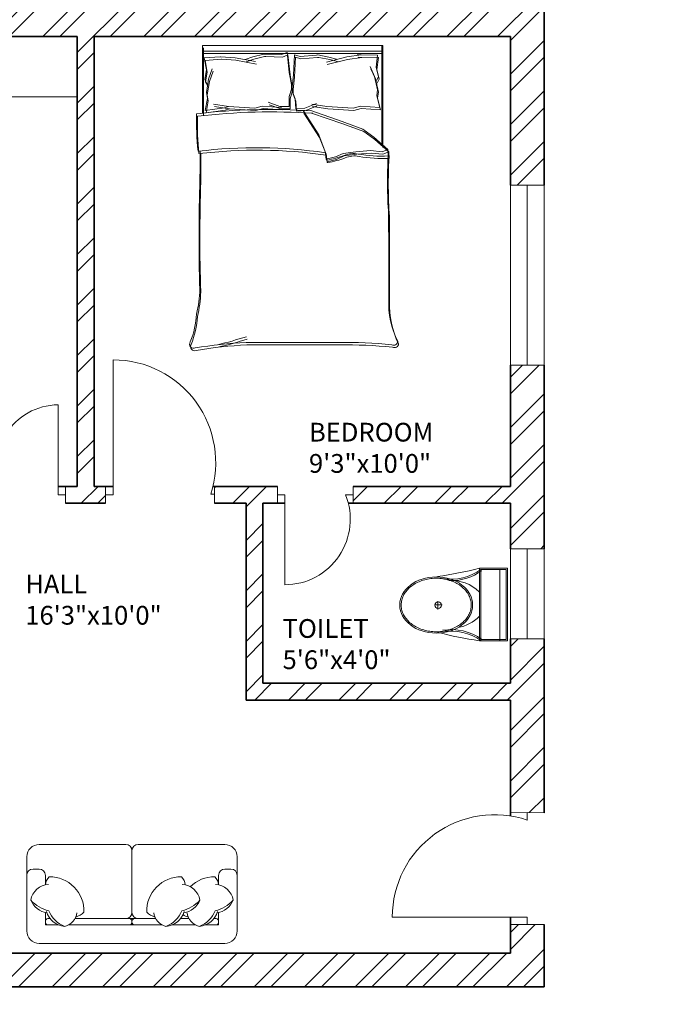
# Model space of a CAD drawing. Units: inches. Extents: x 2552 to 3217, y 1417 to 2737.
# Tile 3 of 25: x 2709 to 2885, y 1622 to 1885. Entities that reach past the tile are written whole.
import ezdxf

# ---------------------------------------------------------------- set-up
doc = ezdxf.new("R2010")
doc.units = ezdxf.units.IN
for name, color, linetype, lineweight in [('A-ANNO-DIMS', 2, 'Continuous', 18), ('A-AREA-IDEN', 7, 'Continuous', 18), ('A-DOOR', 21, 'Continuous', 18), ('A-FLOR-CASE', 9, 'Continuous', 18), ('A-FLOR-FIXT', 8, 'Continuous', 18), ('A-FURN', 8, 'Continuous', 13), ('A-GLAZ', 161, 'Continuous', 18), ('A-WALL', 7, 'Continuous', 35), ('A-WALL-PATT', 217, 'Continuous', 13)]:
    doc.layers.add(name, color=color, linetype=linetype, lineweight=lineweight)
doc.styles.get("Standard").update_dxf_attribs({"font": 'arial.ttf'})
doc.dimstyles.get("Standard").update_dxf_attribs({"dimtxt": 0.18, "dimasz": 0.18, "dimexe": 0.18, "dimexo": 0.0625, "dimgap": 0.09, "dimtad": 0, "dimtih": 1, "dimtoh": 1, "dimdec": 4, "dimzin": 0, "dimdsep": 46, "dimtxsty": 'Standard', "dimcen": 0.09, "dimadec": 0, "dimazin": 0, "dimtfac": 1, "dimtdec": 4, "dimtofl": 0, "dimtmove": 0, "dimatfit": 3, "dimfxl": 1, "dimtolj": 1, "dimtzin": 0, "dimarcsym": 0})

# ---------------------------------------------------------------- blocks, each defined once
blk = doc.blocks.new('A$C31115884')
for p, q in [((283.1, 497.7), (223.4, 497.7)), ((257.5, 466.4), (257.5, 523.2)), ((0, 200), (0, 0)), ((520, 200), (0, 200)), ((10, 190), (10, 10)), ((510, 190), (10, 190)), ((510, 10), (510, 190)), ((520, 0), (520, 200)), ((510, 54.5), (0, 54.5)), ((10, 10), (510, 10)), ((0, 0), (520, 0))]:
    blk.add_line(p, q)
blk.add_circle((255.6, 496.4), 23.6)
for centre, radius, start, end in [((2777.7, -204.6), 2807, 165.4549, 171.71327), ((3237, 905), 2807, 188.28673, 194.5451), ((-294.5, 403.3), 364.7, 324.20913, 9.34987), ((-294.5, 403.3), 374.7, 324.20913, 9.34987), ((805.8, 403.3), 364.7, 170.65013, 215.79087), ((383.6, 406.2), 293.5, 190.27735, 224.15636), ((139.5, 406.2), 293.5, 315.84364, 2.65635), ((805.8, 403.3), 374.7, 179.20365, 215.79087)]:
    blk.add_arc(centre, radius, start, end)
blk.add_ellipse((256.2, 509.9), major_axis=(0, -260.7), ratio=0.772727)
blk.add_open_spline([(256.2, 259.2), (263.1, 259.2), (270, 259.7), (287.8, 262.3), (298.7, 265.1), (319.9, 273.1), (330.2, 278.4), (350.1, 291.1), (359.7, 298.7), (377.7, 315.9), (386.2, 325.5), (401.7, 346.6), (408.8, 358.1), (421.3, 382.5), (426.8, 395.5), (435.9, 422.4), (439.5, 436.4), (444.8, 465.1), (446.5, 479.7), (447.9, 509.2), (447.6, 524), (445, 553.3), (442.7, 567.8), (436.3, 596), (432.1, 609.7), (421.9, 636), (416, 648.6), (402.5, 672.1), (395, 683), (378.6, 703), (369.8, 712.1), (351.1, 728), (341.3, 734.8), (320.9, 746.2), (310.4, 750.7), (288.9, 757.3), (278, 759.4), (256, 761), (245, 760.6), (223.1, 757.2), (212.3, 754.3), (191.1, 746.1), (180.8, 740.7), (160.9, 727.8), (151.4, 720.1), (133.5, 702.7), (125.1, 693), (109.6, 671.7), (102.6, 660.2), (90.2, 635.7), (84.9, 622.7), (76, 595.6), (72.4, 581.6), (67.2, 552.9), (65.6, 538.2), (64.4, 508.8), (64.8, 494), (67.5, 464.7), (69.9, 450.2), (76.6, 422), (80.8, 408.3), (91.1, 382.2), (97.2, 369.7), (110.8, 346.3), (118.4, 335.4), (134.8, 315.6), (143.7, 306.7), (162.4, 290.9), (172.3, 284.2), (192.8, 273), (203.3, 268.6), (224.8, 262.2), (235.8, 260.2), (249.9, 259.3), (253, 259.2), (256.2, 259.2)], degree=3, knots=[0, 0, 0, 0, 0.110105, 0.110105, 0.285049, 0.285049, 0.459994, 0.459994, 0.634938, 0.634938, 0.809882, 0.809882, 0.984827, 0.984827, 1.159771, 1.159771, 1.334715, 1.334715, 1.50966, 1.50966, 1.684604, 1.684604, 1.859549, 1.859549, 2.034493, 2.034493, 2.209437, 2.209437, 2.384382, 2.384382, 2.559326, 2.559326, 2.73427, 2.73427, 2.909215, 2.909215, 3.084159, 3.084159, 3.259103, 3.259103, 3.434048, 3.434048, 3.608992, 3.608992, 3.783936, 3.783936, 3.958881, 3.958881, 4.133825, 4.133825, 4.30877, 4.30877, 4.483714, 4.483714, 4.658658, 4.658658, 4.833603, 4.833603, 5.008547, 5.008547, 5.183491, 5.183491, 5.358436, 5.358436, 5.53338, 5.53338, 5.708324, 5.708324, 5.883269, 5.883269, 6.058213, 6.058213, 6.233158, 6.233158, 6.283185, 6.283185, 6.283185, 6.283185])
blk = doc.blocks.new('BED-DOUBLE')
for p, q in [((3.47, 63.33), (3.47, 81.44)), ((3.47, 81.44), (51.49, 81.44)), ((3.48, 63.33), (3.48, 81.44)), ((51.27, 81.44), (51.27, 54.83)), ((51.27, 81.44), (51.27, 54.83)), ((51.49, 81.44), (51.49, 80.8)), ((3.47, 79.91), (51.27, 79.91)), ((3.48, 79.91), (51.27, 79.91)), ((3.7, 62.69), (3.7, 80.8)), ((3.7, 62.69), (3.7, 80.8)), ((3.7, 79.27), (51.49, 79.27)), ((3.7, 79.27), (51.49, 79.27)), ((16.88, 78.42), (19.77, 79.14)), ((16.88, 78.42), (19.77, 79.14)), ((19.77, 79.14), (20.09, 79.14)), ((19.77, 79.14), (20.09, 79.14)), ((20.09, 79.14), (24.54, 78.99)), ((20.09, 79.14), (24.54, 78.99)), ((24.54, 78.99), (25.98, 79.57)), ((24.54, 78.99), (25.98, 79.57)), ((24.77, 78.36), (26.21, 78.93)), ((24.77, 78.36), (26.21, 78.93)), ((25.98, 79.57), (26.56, 74.22)), ((25.98, 79.57), (26.56, 74.22)), ((26.21, 78.93), (26.79, 73.58)), ((26.21, 78.93), (26.79, 73.58)), ((27.98, 78.95), (27.73, 73.58)), ((27.98, 78.95), (27.73, 73.58)), ((29.46, 78.46), (27.98, 78.95)), ((29.46, 78.46), (27.98, 78.95)), ((33.88, 78.89), (29.46, 78.46)), ((33.88, 78.89), (29.46, 78.46)), ((34.2, 78.91), (33.88, 78.89)), ((34.2, 78.91), (33.88, 78.89)), ((37.14, 78.36), (34.2, 78.91)), ((37.14, 78.36), (34.2, 78.91)), ((45.71, 78.9), (41.91, 78.37)), ((45.71, 78.9), (41.91, 78.37)), ((50.11, 78.89), (44.71, 78.98)), ((44.71, 78.98), (45.71, 78.9)), ((50.11, 78.89), (44.71, 78.98)), ((44.71, 78.98), (45.71, 78.9)), ((50.11, 78.89), (49.73, 75.68)), ((50.11, 78.89), (49.73, 75.68)), ((51.49, 80.8), (51.49, 54.19)), ((51.49, 80.8), (51.49, 54.19)), ((3.89, 78.13), (4.47, 74.95)), ((3.89, 78.13), (4.47, 74.95)), ((3.9, 78.11), (8.18, 78.43)), ((3.9, 78.11), (8.18, 78.43)), ((4.12, 77.49), (4.7, 74.31)), ((4.12, 77.49), (4.7, 74.31)), ((4.13, 77.47), (8.41, 77.8)), ((4.13, 77.47), (8.41, 77.8)), ((8.18, 78.43), (8.28, 78.42)), ((8.18, 78.43), (8.28, 78.42)), ((8.28, 78.42), (12.11, 78.13)), ((8.28, 78.42), (12.11, 78.13)), ((8.41, 77.8), (8.51, 77.78)), ((8.41, 77.8), (8.51, 77.78)), ((8.51, 77.78), (12.34, 77.49)), ((8.51, 77.78), (12.34, 77.49)), ((12.11, 78.13), (17.6, 77.12)), ((12.11, 78.13), (17.6, 77.12)), ((12.34, 77.49), (17.83, 76.48)), ((12.34, 77.49), (17.83, 76.48)), ((14.85, 77.69), (16.88, 78.42)), ((14.85, 77.69), (16.88, 78.42)), ((15.08, 77.05), (17.11, 77.78)), ((15.08, 77.05), (17.11, 77.78)), ((17.11, 77.78), (20, 78.5)), ((17.11, 77.78), (20, 78.5)), ((20, 78.5), (20.32, 78.5)), ((20, 78.5), (20.32, 78.5)), ((20.32, 78.5), (24.77, 78.36)), ((20.32, 78.5), (24.77, 78.36)), ((28.21, 78.31), (27.96, 72.94)), ((28.21, 78.31), (27.96, 72.94)), ((29.68, 77.83), (28.21, 78.31)), ((29.68, 77.83), (28.21, 78.31)), ((34.11, 78.25), (29.68, 77.83)), ((34.11, 78.25), (29.68, 77.83)), ((34.43, 78.27), (34.11, 78.25)), ((34.43, 78.27), (34.11, 78.25)), ((37.36, 77.73), (34.43, 78.27)), ((37.36, 77.73), (34.43, 78.27)), ((41.91, 78.37), (36.49, 77.02)), ((41.91, 78.37), (36.5, 77.02)), ((42.14, 77.73), (36.72, 76.38)), ((42.14, 77.73), (36.72, 76.38)), ((39.2, 77.77), (37.14, 78.36)), ((39.2, 77.77), (37.14, 78.36)), ((39.43, 77.13), (37.36, 77.73)), ((39.43, 77.13), (37.36, 77.73)), ((45.94, 78.26), (42.14, 77.73)), ((45.94, 78.26), (42.14, 77.73)), ((50.34, 78.25), (44.94, 78.34)), ((44.94, 78.34), (45.94, 78.26)), ((50.34, 78.25), (44.94, 78.34)), ((44.94, 78.34), (45.94, 78.26)), ((50.34, 78.25), (49.96, 75.04)), ((50.34, 78.25), (49.96, 75.04)), ((4.47, 74.95), (4.04, 72.34)), ((4.47, 74.95), (4.04, 72.34)), ((4.7, 74.31), (4.27, 71.7)), ((4.7, 74.31), (4.27, 71.7)), ((5.05, 72.49), (6.06, 75.24)), ((5.05, 72.49), (6.06, 75.24)), ((5.28, 71.85), (6.29, 74.6)), ((5.28, 71.85), (6.29, 74.6)), ((26.56, 74.22), (27.14, 71.04)), ((26.56, 74.22), (27.14, 71.04)), ((26.79, 73.58), (27.37, 70.4)), ((26.79, 73.58), (27.37, 70.4)), ((27.73, 73.58), (27.35, 70.37)), ((27.73, 73.58), (27.35, 70.37)), ((49.31, 73.19), (48.13, 75.86)), ((49.31, 73.19), (48.13, 75.86)), ((49.54, 72.55), (48.36, 75.23)), ((49.54, 72.55), (48.36, 75.23)), ((49.73, 75.68), (50.33, 73.1)), ((49.73, 75.68), (50.33, 73.1)), ((49.96, 75.04), (50.56, 72.47)), ((49.96, 75.04), (50.56, 72.47)), ((4.04, 72.34), (4.62, 71.33)), ((4.04, 72.34), (4.62, 71.33)), ((4.27, 71.7), (4.85, 70.69)), ((4.27, 71.7), (4.85, 70.69)), ((4.47, 68.87), (5.05, 72.49)), ((4.47, 68.87), (5.05, 72.49)), ((4.7, 68.23), (5.28, 71.85)), ((4.7, 68.23), (5.28, 71.85)), ((27.14, 71.04), (27.14, 69.74)), ((27.14, 71.04), (27.14, 69.74)), ((27.96, 72.94), (27.58, 69.73)), ((27.96, 72.94), (27.58, 69.73)), ((50.11, 69.61), (49.31, 73.19)), ((50.11, 69.61), (49.31, 73.19)), ((50.34, 68.98), (49.54, 72.55)), ((50.34, 68.98), (49.54, 72.55)), ((50.33, 73.1), (49.81, 72.06)), ((50.33, 73.1), (49.81, 72.06)), ((50.56, 72.47), (50.04, 71.42)), ((50.56, 72.47), (50.04, 71.42)), ((4.76, 67.28), (4.47, 68.87)), ((4.76, 67.28), (4.47, 68.87)), ((27.14, 69.74), (26.56, 67.86)), ((27.14, 69.74), (26.56, 67.86)), ((27.37, 69.1), (26.79, 67.22)), ((27.37, 69.1), (26.79, 67.22)), ((27.35, 70.37), (27.44, 69.07)), ((27.35, 70.37), (27.44, 69.07)), ((27.37, 70.4), (27.37, 69.1)), ((27.37, 70.4), (27.37, 69.1)), ((27.44, 69.07), (28.13, 67.23)), ((27.44, 69.07), (28.13, 67.23)), ((27.58, 69.73), (27.66, 68.43)), ((27.58, 69.73), (27.66, 68.43)), ((27.66, 68.43), (28.36, 66.59)), ((27.66, 68.43), (28.36, 66.59)), ((49.92, 68.01), (50.11, 69.61)), ((49.92, 68.01), (50.11, 69.61)), ((50.15, 67.37), (50.34, 68.98)), ((50.15, 67.37), (50.34, 68.98)), ((4.18, 64.1), (4.76, 67.28)), ((4.18, 64.1), (4.76, 67.28)), ((4.41, 63.46), (4.99, 66.64)), ((4.41, 63.46), (4.99, 66.64)), ((4.99, 66.64), (4.7, 68.23)), ((4.99, 66.64), (4.7, 68.23)), ((6.38, 65.81), (10.41, 65.15)), ((6.38, 65.81), (10.41, 65.15)), ((24.1, 65.18), (20.96, 66.27)), ((24.1, 65.18), (20.96, 66.27)), ((26.56, 67.86), (26.56, 65.18)), ((26.56, 67.86), (26.56, 65.18)), ((26.79, 67.22), (26.79, 64.54)), ((26.79, 67.22), (26.79, 64.54)), ((28.13, 67.23), (28.3, 64.55)), ((28.13, 67.23), (28.3, 64.55)), ((28.36, 66.59), (28.53, 63.91)), ((28.36, 66.59), (28.53, 63.91)), ((30.75, 64.7), (33.82, 65.99)), ((30.75, 64.7), (33.82, 65.99)), ((32.56, 65.81), (36.6, 65.15)), ((32.56, 65.81), (36.6, 65.15)), ((50.7, 64.87), (49.92, 68.01)), ((50.7, 64.87), (49.92, 68.01)), ((50.93, 64.23), (50.15, 67.37)), ((50.93, 64.23), (50.15, 67.37)), ((9.28, 64.83), (4.18, 64.1)), ((9.28, 64.83), (4.18, 64.1)), ((9.51, 64.19), (4.41, 63.46)), ((9.51, 64.19), (4.41, 63.46)), ((6.61, 65.18), (10.64, 64.51)), ((6.61, 65.18), (10.64, 64.51)), ((10.41, 65.15), (9.28, 64.83)), ((10.41, 65.15), (9.28, 64.83)), ((10.64, 64.51), (9.51, 64.19)), ((10.64, 64.51), (9.51, 64.19)), ((10.41, 65.15), (17.42, 64.72)), ((10.41, 65.15), (17.42, 64.72)), ((10.64, 64.51), (17.65, 64.08)), ((10.64, 64.51), (17.65, 64.08)), ((17.42, 64.72), (19.38, 65.27)), ((17.42, 64.72), (19.38, 65.27)), ((17.65, 64.08), (19.61, 64.63)), ((17.65, 64.08), (19.61, 64.63)), ((19.38, 65.27), (24.52, 64.87)), ((19.38, 65.27), (24.52, 64.87)), ((19.61, 64.63), (24.74, 64.23)), ((19.61, 64.63), (24.74, 64.23)), ((24.33, 64.54), (21.19, 65.63)), ((24.33, 64.54), (21.19, 65.63)), ((26.56, 65.18), (24.1, 65.18)), ((26.56, 65.18), (24.1, 65.18)), ((26.79, 64.54), (24.33, 64.54)), ((26.79, 64.54), (24.33, 64.54)), ((28.3, 64.55), (30.75, 64.7)), ((28.3, 64.55), (30.75, 64.7)), ((28.53, 63.91), (30.98, 64.06)), ((28.53, 63.91), (30.98, 64.06)), ((30.26, 64.06), (34.45, 57.57)), ((30.26, 64.06), (34.45, 57.57)), ((30.49, 63.42), (34.68, 56.93)), ((30.49, 63.42), (34.68, 56.93)), ((30.98, 64.06), (34.05, 65.35)), ((30.98, 64.06), (34.05, 65.35)), ((40.64, 61.13), (32.31, 64.06)), ((40.64, 61.13), (32.31, 64.06)), ((40.87, 60.49), (32.53, 63.42)), ((40.87, 60.49), (32.53, 63.42)), ((32.79, 65.18), (36.82, 64.51)), ((32.79, 65.18), (36.82, 64.51)), ((36.6, 65.15), (43.61, 64.72)), ((36.6, 65.15), (43.61, 64.72)), ((36.82, 64.51), (43.83, 64.08)), ((36.82, 64.51), (43.83, 64.08)), ((43.61, 64.72), (45.57, 65.27)), ((43.61, 64.72), (45.57, 65.27)), ((43.83, 64.08), (45.79, 64.63)), ((43.83, 64.08), (45.79, 64.63)), ((45.57, 65.27), (50.7, 64.87)), ((45.57, 65.27), (50.7, 64.87)), ((45.79, 64.63), (50.93, 64.23)), ((45.79, 64.63), (50.93, 64.23)), ((46.22, 59.11), (40.64, 61.13)), ((46.22, 59.11), (40.64, 61.13)), ((46.45, 58.48), (40.87, 60.49)), ((46.45, 58.48), (40.87, 60.49)), ((49.16, 56.95), (46.22, 59.11)), ((49.16, 56.95), (46.22, 59.11)), ((49.39, 56.31), (46.45, 58.48)), ((49.39, 56.31), (46.45, 58.48)), ((34.45, 57.57), (36.15, 53.08)), ((34.45, 57.57), (36.15, 53.08)), ((34.68, 56.93), (36.38, 52.44)), ((34.68, 56.93), (36.38, 52.44)), ((52.87, 53.7), (49.16, 56.95)), ((52.87, 53.7), (49.16, 56.95)), ((53.1, 53.06), (49.39, 56.31)), ((53.1, 53.06), (49.39, 56.31)), ((36.15, 53.08), (36.46, 51.07)), ((36.15, 53.08), (36.46, 51.07)), ((38.94, 51.69), (40.95, 52.61)), ((38.94, 51.69), (40.95, 52.61)), ((40.95, 52.61), (44.36, 53.08)), ((40.95, 52.61), (44.36, 53.08)), ((44.36, 53.08), (48.23, 53.39)), ((44.36, 53.08), (48.23, 53.39)), ((44.59, 52.44), (48.46, 52.75)), ((44.59, 52.44), (48.46, 52.75)), ((48.23, 53.39), (51.33, 53.08)), ((48.23, 53.39), (51.33, 53.08)), ((48.46, 52.75), (51.56, 52.44)), ((48.46, 52.75), (51.56, 52.44)), ((51.33, 53.08), (52.87, 53.7)), ((51.33, 53.08), (52.87, 53.7)), ((51.56, 52.44), (53.1, 53.06)), ((51.56, 52.44), (53.1, 53.06)), ((52.95, 51.95), (52.87, 53.7, 3.87)), ((52.95, 51.95), (52.87, 53.7, 3.87)), ((53.18, 51.31), (53.1, 53.06, 3.87)), ((53.18, 51.31), (53.1, 53.06, 3.87)), ((36.38, 52.44), (36.69, 50.43)), ((36.38, 52.44), (36.69, 50.43)), ((36.46, 51.07), (38.94, 51.69)), ((36.46, 51.07), (38.94, 51.69)), ((36.69, 50.43), (39.17, 51.05)), ((36.69, 50.43), (39.17, 51.05)), ((39.17, 51.05), (41.18, 51.97)), ((39.17, 51.05), (41.18, 51.97)), ((41.18, 51.97), (44.59, 52.44)), ((41.18, 51.97), (44.59, 52.44)), ((15.06, 2.2), (39.68, 2.2)), ((15.06, 2.2), (39.68, 2.2)), ((15.29, 1.56), (39.91, 1.56)), ((15.29, 1.56), (39.91, 1.56))]:
    blk.add_line(p, q)
for centre, radius, start, end in [((85.16, 61.35), 83.31, 178.7218, 185.604), ((85.16, 61.35), 83.31, 178.7218, 185.604), ((21.36, -100.61), 164.97, 86.0865, 96.7821), ((21.36, -100.61), 164.97, 86.0865, 96.7821), ((21.59, -101.25), 164.97, 86.0865, 96.7821), ((21.59, -101.25), 164.97, 86.0865, 96.7821), ((85.39, 60.71), 83.31, 178.7218, 185.604), ((85.39, 60.71), 83.31, 178.7218, 185.604), ((17.76, -74.87), 129.02, 81.7845, 96.9006), ((17.76, -74.87), 129.02, 81.7845, 96.9006), ((17.98, -75.51), 129.02, 81.7845, 96.9006), ((17.98, -75.51), 129.02, 81.7845, 96.9006), ((-167.31, 50.27), 170.11, 358.4762, 1.0082), ((-167.31, 50.27), 170.11, 358.4762, 1.0082), ((-167.08, 49.63), 170.11, 358.4762, 1.0082), ((-167.08, 49.63), 170.11, 358.4762, 1.0082), ((43.74, 46.38), 6.22, 78.6608, 113.7384), ((43.74, 46.38), 6.22, 78.6608, 113.7384), ((36.64, 51), 0.185, 160.2464, 271.1377), ((36.64, 51), 0.185, 160.2464, 271.1377), ((31.15, 79.96), 29.65, 280.6617, 289.8806), ((31.15, 79.96), 29.65, 280.6617, 289.8806), ((36.86, 50.36), 0.185, 160.2464, 271.1377), ((36.86, 50.36), 0.185, 160.2464, 271.1377), ((31.38, 79.32), 29.65, 280.6617, 289.8806), ((31.38, 79.32), 29.65, 280.6617, 289.8806), ((43.97, 45.74), 6.22, 78.6608, 113.7384), ((43.97, 45.74), 6.22, 78.6608, 113.7384), ((51.33, 88.1), 36.18, 259.8763, 272.5657), ((51.33, 88.1), 36.18, 259.8763, 272.5657), ((51.56, 87.46), 36.18, 259.8763, 272.5657), ((51.56, 87.46), 36.18, 259.8763, 272.5657), ((182.27, 45.13), 129.5, 176.9791, 183.8365), ((182.27, 45.13), 129.5, 176.9791, 183.8365), ((182.49, 44.49), 129.5, 176.9791, 183.8365), ((182.49, 44.49), 129.5, 176.9791, 183.8365), ((484.82, 30.83), 482.31, 178.2277, 181.7185), ((484.82, 30.83), 482.31, 178.2277, 181.7185), ((485.05, 30.19), 482.31, 178.2277, 181.7185), ((485.05, 30.19), 482.31, 178.2277, 181.7185), ((-4508.74, 13.62), 4561.86, 0.00217, 0.28689), ((-4508.74, 13.62), 4561.86, 0.00217, 0.28689), ((-4508.51, 12.98), 4561.86, 0.00217, 0.28689), ((-4508.52, 12.98), 4561.86, 0.00217, 0.28689), ((-26.9, 16.93), 29.63, 346.0648, 358.9113), ((-26.9, 16.93), 29.63, 346.0648, 358.9113), ((-26.67, 16.29), 29.63, 346.0648, 358.9113), ((-26.67, 16.29), 29.63, 346.0648, 358.9113), ((76.16, 12.78), 23.07, 177.4714, 206.4681), ((76.16, 12.78), 23.07, 177.4714, 206.4681), ((76.39, 12.14), 23.07, 177.4714, 206.4681), ((76.39, 12.14), 23.07, 177.4714, 206.4681), ((-21.66, 11.17), 23.56, 337.9751, 356.652), ((-21.66, 11.17), 23.56, 337.9751, 356.652), ((-21.43, 10.53), 23.56, 337.9751, 356.652), ((-21.43, 10.53), 23.56, 337.9751, 356.652), ((-17.22, 105.16), 106.46, 283.3832, 287.7053), ((-17.22, 105.16), 106.46, 283.3832, 287.7053), ((-16.99, 104.52), 106.46, 283.3832, 287.7053), ((-16.99, 104.52), 106.46, 283.3832, 287.7053), ((1.09, 1.73), 1.09, 146.1736, 293.4781), ((1.09, 1.73), 1.09, 146.1736, 293.4781), ((1.32, 1.09), 1.09, 146.1736, 293.4781), ((1.32, 1.09), 1.09, 146.1736, 293.4781), ((21.43, -119.39), 121.76, 92.9958, 99.4091), ((21.43, -119.39), 121.76, 92.9958, 99.4091), ((21.66, -120.03), 121.76, 92.9958, 99.4091), ((21.65, -120.03), 121.76, 92.9958, 99.4091), ((41.15, -130.83), 133.04, 84.4998, 90.6351), ((41.15, -130.83), 133.04, 84.4998, 90.6351), ((41.38, -131.47), 133.04, 84.4998, 90.6351), ((41.38, -131.47), 133.04, 84.4998, 90.6351), ((54.41, 2.57), 1.1, 242.6588, 356.02), ((54.41, 2.57), 1.1, 242.6588, 356.02), ((54.64, 1.93), 1.1, 242.6588, 356.02), ((54.64, 1.93), 1.1, 242.6588, 356.02)]:
    blk.add_arc(centre, radius, start, end)
blk = doc.blocks.new('WIN-48')
for p, q in [((4.5, 48), (0, 48)), ((0, 48), (9, 48)), ((0, 48), (0, 0)), ((4.5, 0), (4.5, 48)), ((9, 48), (9, 0)), ((0, 0), (9, 0)), ((9, 0), (4.5, 0))]:
    blk.add_line(p, q)
blk = doc.blocks.new('*D64')
at = {"layer": 'A-ANNO-DIMS', "color": 0, "lineweight": -2, "transparency": 16777216}
for p, q in [((2646.35, 1551.58), (2646.35, 2709.49)), ((2646.53, 2709.31), (2802.77, 2709.31)), ((2959.93, 2709.31), (2803.69, 2709.31)), ((2960.11, 1551.58), (2960.11, 2709.49))]:
    blk.add_line(p, q, dxfattribs=at)
at = {"layer": 'A-ANNO-DIMS', "color": 0, "transparency": 16777216}
for points in [[(2646.53, 2709.34), (2646.53, 2709.28), (2646.35, 2709.31)], [(2959.93, 2709.34), (2959.93, 2709.28), (2960.11, 2709.31)]]:
    blk.add_solid(points, dxfattribs=at)
at = {"layer": 'Defpoints', "color": 0, "transparency": 16777216}
for p in [(2960.11, 2709.31), (2646.35, 1551.51), (2960.11, 1551.51)]:
    blk.add_point(p, dxfattribs=at)
at = {"layer": 'A-ANNO-DIMS', "color": 0, "transparency": 16777216, "insert": (2803.23, 2709.31), "char_height": 0.18, "attachment_point": 5}
blk.add_mtext('\\A1;313.76', dxfattribs=at)

msp = doc.modelspace()

# ---------------------------------------------------------------- hatches: boundary and pattern name
at = {"layer": 'A-WALL-PATT'}
h = msp.add_hatch(dxfattribs=at)
h.set_pattern_fill('ANSI32', color=256)
h.paths.add_polyline_path([(2756.676, 2649.5125), (2637.3535, 2649.5125), (2637.3535, 2617.9626), (2641.8535, 2617.9626), (2646.3535, 2617.9626), (2646.3535, 2640.5125), (2724.3535, 2640.5125), (2724.3535, 2520.5125), (2720.299, 2520.5125), (2720.299, 2516.0125), (2733.4075, 2516.0125), (2733.4075, 2518.2213), (2733.4075, 2520.5125), (2728.8535, 2520.5125), (2728.8535, 2640.5125), (2756.676, 2640.5125)])
h.paths.add_polyline_path([(2848.8535, 2649.5125), (2804.676, 2649.5125), (2804.676, 2640.5125), (2839.8535, 2640.5125), (2839.8535, 2598.3517), (2848.8535, 2598.3517)])
h.paths.add_polyline_path([(2646.3535, 2516.0125), (2697.9593, 2516.0125), (2697.9593, 2518.2625), (2697.9593, 2520.5125), (2646.3535, 2520.5125), (2646.3535, 2581.9626), (2637.3535, 2581.9626), (2637.3535, 2364.3298), (2646.3535, 2364.3298), (2646.3535, 2387.0125), (2724.3535, 2387.0125), (2724.3535, 2267.0125), (2721.0443, 2267.0125), (2721.0443, 2262.5125), (2733.7854, 2262.5125), (2733.7854, 2264.7625), (2733.7854, 2267.0125), (2728.8535, 2267.0125), (2728.8535, 2387.0125), (2839.8535, 2387.0125), (2839.8535, 2363.8387), (2848.8535, 2363.8387), (2848.8535, 2403.7415), (2844.3535, 2403.7415), (2839.8535, 2403.7415), (2839.8535, 2396.0125), (2646.3535, 2396.0125)])
h.paths.add_polyline_path([(2848.8535, 2550.3517), (2844.3535, 2550.3517), (2839.8535, 2550.3517), (2839.8535, 2520.5125), (2801.9195, 2520.5125), (2801.9195, 2518.2625), (2801.9195, 2516.0125), (2839.8535, 2516.0125), (2839.8535, 2507.5813), (2848.8535, 2507.5813)], flags=17)
h.paths.add_polyline_path([(2848.8535, 2483.5813), (2844.3535, 2483.5813), (2839.8535, 2483.5813), (2839.8535, 2468.0125), (2773.8535, 2468.0125), (2773.8535, 2516.0125), (2778.1336, 2516.0125), (2778.1336, 2520.5125), (2766.696, 2520.5125), (2766.696, 2518.2625), (2766.696, 2516.0125), (2769.3535, 2516.0125), (2769.3535, 2463.5125), (2839.8535, 2463.5125), (2839.8535, 2431.0782), (2848.8535, 2431.0782)], flags=17)
h.paths.add_polyline_path([(2917.8535, 2569.2764), (2913.3535, 2569.2764), (2908.8535, 2569.2764), (2908.8535, 2433.001), (2917.8535, 2433.001), (2917.8535, 2516.0125), (2967.486, 2516.0125), (2967.486, 2520.5125), (2917.8535, 2520.5125)])
h.paths.add_polyline_path([(3000.3535, 2640.5125), (2995.8535, 2640.5125), (2995.8535, 2520.5125), (2990.688, 2520.5125), (2990.688, 2516.0125), (3004.0844, 2516.0125), (3004.0844, 2518.2625), (3004.0844, 2520.5125), (3000.3535, 2520.5125)])
h.paths.add_polyline_path([(3120.3535, 2561.3689), (3115.8535, 2561.3689), (3111.3535, 2561.3689), (3111.3535, 2520.5125), (3070.9814, 2520.5125), (3070.9814, 2518.2625), (3070.9814, 2516.0125), (3111.3535, 2516.0125), (3111.3535, 2505.1841), (3120.3535, 2505.1841)])
h.paths.add_polyline_path([(3120.3535, 2481.1841), (3115.8535, 2481.1841), (3111.3535, 2481.1841), (3111.3535, 2468.0125), (3045.3535, 2468.0125), (3045.3535, 2516.0125), (3048.9787, 2516.0125), (3048.9787, 2520.5125), (3036.3395, 2520.5125), (3036.3395, 2516.0125), (3040.8535, 2516.0125), (3040.8535, 2463.5125), (3111.3535, 2463.5125), (3111.3535, 2396.0125), (2917.8535, 2396.0125), (2917.8535, 2403.4124), (2913.3535, 2403.4124), (2908.8535, 2403.4124), (2908.8535, 2182.5756), (2917.8535, 2182.5756), (2917.8535, 2262.5125), (2968.001, 2262.5125), (2968.001, 2264.7625), (2968.001, 2267.0125), (2917.8535, 2267.0125), (2917.8535, 2387.0125), (3111.3535, 2387.0125), (3111.3535, 2352.2435), (3120.3535, 2352.2435)])
h.paths.add_polyline_path([(3120.3535, 2304.2435), (3115.8535, 2304.2435), (3111.3535, 2304.2435), (3111.3535, 2267.0125), (3073.8616, 2267.0125), (3073.8616, 2264.7625), (3073.8616, 2262.5125), (3111.3535, 2262.5125), (3111.3535, 2252.376), (3120.3535, 2252.376)], flags=17)
h.paths.add_polyline_path([(3120.3535, 2228.376), (3115.8535, 2228.376), (3111.3535, 2228.376), (3111.3535, 2214.5125), (3045.3535, 2214.5125), (3045.3535, 2262.5125), (3049.3096, 2262.5125), (3049.3096, 2267.0125), (3035.0125, 2267.0125), (3035.0125, 2262.5125), (3040.8535, 2262.5125), (3040.8535, 2210.0125), (3111.3535, 2210.0125), (3111.3535, 2142.5125), (2917.8535, 2142.5125), (2917.8535, 2150.2408), (2913.3535, 2150.2408), (2908.8535, 2150.2408), (2908.8535, 1924.9905), (2917.8535, 1924.9905), (2917.8535, 2009.0125), (2971.959, 2009.0125), (2971.959, 2011.2625), (2971.959, 2013.5125), (2917.8535, 2013.5125), (2917.8535, 2133.5125), (2995.8535, 2133.5125), (2995.8535, 2013.5125), (2992.1797, 2013.5125), (2992.1797, 2009.0125), (3004.3344, 2009.0125), (3004.3344, 2011.2625), (3004.3344, 2013.5125), (3000.3535, 2013.5125), (3000.3535, 2133.5125), (3111.3535, 2133.5125), (3111.3535, 2115.0291), (3120.3535, 2115.0291)])
h.paths.add_polyline_path([(3000.3535, 2387.0125), (2995.8535, 2387.0125), (2995.8535, 2267.0125), (2991.3326, 2267.0125), (2991.3326, 2262.5125), (3004.1044, 2262.5125), (3004.1044, 2264.7625), (3004.1044, 2267.0125), (3000.3535, 2267.0125)], flags=17)
h.paths.add_polyline_path([(3120.3535, 1973.2388), (3115.8535, 1973.2388), (3111.3535, 1973.2388), (3111.3535, 1961.0125), (3045.3535, 1961.0125), (3045.3535, 2009.0125), (3048.9101, 2009.0125), (3048.9101, 2013.5125), (3037.105, 2013.5125), (3037.105, 2011.2625), (3037.105, 2009.0125), (3040.8535, 2009.0125), (3040.8535, 1956.5125), (3111.3535, 1956.5125), (3111.3535, 1889.0125), (2917.8535, 1889.0125), (2917.8535, 1895.7215), (2913.3535, 1895.7215), (2908.8535, 1895.7215), (2908.8535, 1844.2217), (2917.8535, 1844.2217), (2917.8535, 1880.0125), (3111.3535, 1880.0125), (3111.3535, 1846.9541), (3120.3535, 1846.9541)])
h.paths.add_polyline_path([(3120.3535, 2067.0291), (3111.3535, 2067.0291), (3111.3535, 2013.5125), (3071.3001, 2013.5125), (3071.3001, 2009.0125), (3111.3535, 2009.0125), (3111.3535, 1997.2388), (3120.3535, 1997.2388)], flags=0)
h.paths.add_polyline_path([(3120.3535, 1798.9541), (3115.8535, 1798.9541), (3111.3535, 1798.9541), (3111.3535, 1760.0125), (3071.2497, 1760.0125), (3071.2497, 1757.7625), (3071.2497, 1755.5125), (3111.3535, 1755.5125), (3111.3535, 1746.162), (3120.3535, 1746.2478)])
h.paths.add_polyline_path([(3120.3535, 1722.2049), (3111.3535, 1722.2049), (3111.3535, 1707.5125), (3045.3535, 1707.5125), (3045.3535, 1755.5125), (3048.6624, 1755.5125), (3048.6624, 1760.0125), (3035.3703, 1760.0125), (3035.3703, 1755.5125), (3040.8535, 1755.5125), (3040.8535, 1703.0125), (3111.3535, 1703.0125), (3111.3535, 1635.5125), (2917.8535, 1635.5125), (2917.8535, 1643.1366), (2913.3535, 1643.1366), (2908.8535, 1643.1366), (2908.8535, 1626.5125), (3120.3535, 1626.5125)])
h.paths.add_polyline_path([(2917.8535, 1755.5125), (2973.2287, 1755.5125), (2973.2287, 1757.7625), (2973.2287, 1760.0125), (2917.8535, 1760.0125), (2917.8535, 1808.2217), (2913.3535, 1808.2217), (2908.8535, 1808.2217), (2908.8535, 1676.1665), (2917.8535, 1676.1665)])
h.paths.add_polyline_path([(3000.3535, 1880.0125), (2995.8535, 1880.0125), (2995.8535, 1760.0125), (2992.9329, 1760.0125), (2992.9329, 1755.5125), (3003.8766, 1755.5125), (3003.8766, 1757.7625), (3003.8766, 1760.0125), (3000.3535, 1760.0125)])
h.paths.add_polyline_path([(2848.8535, 1896.6971), (2844.3535, 1896.6971), (2839.8535, 1896.6971), (2839.8535, 1889.0125), (2646.3535, 1889.0125), (2646.3535, 2009.0125), (2700.5253, 2009.0125), (2700.5253, 2011.2625), (2700.5253, 2013.5125), (2646.3535, 2013.5125), (2646.3535, 2053.1812), (2641.8535, 2053.1812), (2637.3535, 2053.1812), (2637.3535, 1836.254), (2646.3535, 1836.254), (2646.3535, 1880.0125), (2724.3535, 1880.0125), (2724.3535, 1760.0125), (2721.2473, 1760.0125), (2721.2473, 1755.5125), (2731.9187, 1755.5125), (2731.9187, 1757.7625), (2731.9187, 1760.0125), (2728.8535, 1760.0125), (2728.8535, 1880.0125), (2839.8535, 1880.0125), (2839.8535, 1840.3813), (2848.8535, 1840.3813)])
h.paths.add_polyline_path([(2848.8535, 1792.3813), (2844.3535, 1792.3813), (2839.8535, 1792.3813), (2839.8535, 1760.0125), (2797.8845, 1760.0125), (2797.8845, 1755.5125), (2839.8535, 1755.5125), (2839.8535, 1743.3688), (2844.3535, 1743.3688), (2848.8535, 1743.3688)], flags=0)
h.paths.add_polyline_path([(2848.8535, 1719.3688), (2844.3535, 1719.3688), (2839.8535, 1719.3688), (2839.8535, 1707.5125), (2773.8535, 1707.5125), (2773.8535, 1755.5125), (2777.716, 1755.5125), (2777.716, 1760.0125), (2760.9247, 1760.0125), (2760.9247, 1757.9721), (2760.9247, 1755.5125), (2769.3535, 1755.5125), (2769.3535, 1703.0125), (2839.8535, 1703.0125), (2839.8535, 1673.0277), (2848.8535, 1672.9407)], flags=0)
h.paths.add_polyline_path([(2646.3535, 1755.5125), (2702.9171, 1755.5125), (2702.9171, 1757.7625), (2702.9171, 1760.0125), (2646.3535, 1760.0125), (2646.3535, 1800.254), (2641.8535, 1800.254), (2637.3535, 1800.254), (2637.3535, 1626.5125), (2848.8535, 1626.5125), (2848.8535, 1643.1187), (2844.3535, 1643.1187), (2839.8535, 1643.1187), (2839.8535, 1635.5125), (2646.3535, 1635.5125)])
h.paths.add_polyline_path([(2848.8535, 2148.8427), (2844.3535, 2148.8427), (2839.8535, 2148.8427), (2839.8535, 2142.5125), (2646.3535, 2142.5125), (2646.3535, 2262.5125), (2701.3562, 2262.5125), (2701.3562, 2264.7625), (2701.3562, 2267.0125), (2646.3535, 2267.0125), (2646.3535, 2328.3298), (2637.3535, 2328.3298), (2637.3535, 2089.1812), (2646.3535, 2089.1812), (2646.3535, 2133.5125), (2839.8535, 2133.5125), (2839.8535, 2097.5966), (2848.8535, 2097.5966)])
h.paths.add_polyline_path([(2728.8535, 2133.5125), (2724.3535, 2133.5125), (2724.3535, 2013.5125), (2719.6039, 2013.5125), (2719.6039, 2009.0125), (2732.5784, 2009.0125), (2732.5784, 2011.2625), (2732.5784, 2013.5125), (2728.8535, 2013.5125)])
h.paths.add_polyline_path([(2848.8535, 1970.0557), (2844.3535, 1970.0557), (2839.8535, 1970.0557), (2839.8535, 1961.0125), (2773.8535, 1961.0125), (2773.8535, 2009.0125), (2777.3388, 2009.0125), (2777.3388, 2013.5125), (2764.7681, 2013.5125), (2764.7681, 2009.0125), (2769.3535, 2009.0125), (2769.3535, 1956.5125), (2839.8535, 1956.5125), (2839.8535, 1924.7199), (2848.8535, 1924.7199)], flags=17)
h.paths.add_polyline_path([(2848.8535, 2049.5966), (2844.3535, 2049.5966), (2839.8535, 2049.5966), (2839.8535, 2013.5125), (2798.198, 2013.5125), (2798.198, 2011.2625), (2798.198, 2009.0125), (2839.8535, 2009.0125), (2839.8535, 1994.0557), (2848.8535, 1994.0557)], flags=17)
h.paths.add_polyline_path([(2848.8535, 2315.8387), (2839.8535, 2315.8387), (2839.8535, 2267.0125), (2799.3375, 2267.0125), (2799.3375, 2264.7625), (2799.3375, 2262.5125), (2839.8535, 2262.5125), (2839.8535, 2253.2843), (2848.8535, 2253.2843)], flags=17)
h.paths.add_polyline_path([(2848.8535, 2229.2843), (2839.8535, 2229.2843), (2839.8535, 2177.6936), (2848.8535, 2177.6936)], flags=17)
h.paths.add_polyline_path([(2839.8535, 2214.5125), (2773.8535, 2214.5125), (2773.8535, 2262.5125), (2777.6984, 2262.5125), (2777.6984, 2267.0125), (2763.8226, 2267.0125), (2763.8226, 2262.5125), (2769.3535, 2262.5125), (2769.3535, 2210.0125), (2839.8535, 2210.0125)], flags=17)
h.paths.add_polyline_path([(3050.32, 2520.2817), (3088.9114, 2520.2817), (3088.9114, 2538.939), (3050.32, 2538.939)], flags=9)
h = msp.add_hatch(dxfattribs=at)
h.set_pattern_fill('ANSI32', color=256)
h.paths.add_polyline_path([(2848.8535, 1792.3813), (2844.3535, 1792.3813), (2839.8535, 1792.3813), (2839.8535, 1760.0125), (2797.8845, 1760.0125), (2797.8845, 1755.5125), (2839.8535, 1755.5125), (2839.8535, 1743.3688), (2844.3535, 1743.3688), (2848.8535, 1743.3688)])
h.paths.add_polyline_path([(2848.8535, 1719.3688), (2844.3535, 1719.3688), (2839.8535, 1719.3688), (2839.8535, 1707.5125), (2773.8535, 1707.5125), (2773.8535, 1755.5125), (2777.716, 1755.5125), (2777.716, 1760.0125), (2760.9247, 1760.0125), (2760.9247, 1757.9721), (2760.9247, 1755.5125), (2769.3535, 1755.5125), (2769.3535, 1703.0125), (2839.8535, 1703.0125), (2839.8535, 1673.0277), (2848.8535, 1672.9407)])

# ---------------------------------------------------------------- linework, layer by layer
at = {"layer": 'A-DOOR'}
for p, q in [((2733.9187, 1757.7625), (2733.9187, 1793.7625)), ((2719.2473, 1757.7625), (2719.2473, 1781.7625)), ((2721.2473, 1760.0125), (2721.2473, 1755.5125)), ((2731.9187, 1760.0125), (2731.9187, 1755.5125)), ((2760.9247, 1758.8473), (2760.9247, 1760.0125)), ((2760.9247, 1760.0125), (2760.9247, 1757.9721)), ((2777.716, 1755.5125), (2777.716, 1760.0125)), ((2777.716, 1760.0125), (2777.716, 1757.7625)), ((2797.8845, 1760.0125), (2797.8845, 1755.5125)), ((2721.2473, 1757.7625), (2719.2473, 1757.7625)), ((2721.2473, 1755.5125), (2721.2473, 1757.7625)), ((2731.9187, 1755.5125), (2731.9187, 1757.7625)), ((2731.9187, 1757.7625), (2733.9187, 1757.7625)), ((2760.9247, 1757.9721), (2759.9247, 1757.9721)), ((2760.9247, 1755.5125), (2760.9247, 1758.8473)), ((2777.716, 1757.7625), (2779.716, 1757.7625)), ((2779.716, 1757.7625), (2779.716, 1733.7625)), ((2797.8845, 1757.7625), (2795.8845, 1757.7625)), ((2797.8845, 1755.5125), (2797.8845, 1757.7625)), ((2839.8535, 1673.0277), (2848.8535, 1672.9407)), ((2848.8535, 1672.9407), (2844.3535, 1672.9842)), ((2844.3535, 1672.9842), (2844.3535, 1670.9842)), ((2844.3535, 1645.1187), (2808.3535, 1645.1187)), ((2844.3535, 1643.1187), (2844.3535, 1645.1187)), ((2839.8535, 1643.1187), (2848.8535, 1643.1187)), ((2848.8535, 1643.1187), (2844.3535, 1643.1187))]:
    msp.add_line(p, q, dxfattribs=at)
for centre, radius, start, end in [((2733.9187, 1766.4191), 27.3435, 342.005775, 90), ((2719.2473, 1765.4843), 16.2782, 90, 208.31787), ((2779.716, 1751.2088), 17.4463, 270, 22.064484), ((2835.6455, 1645.1187), 27.292, 71.393314, 180)]:
    msp.add_arc(centre, radius, start, end, dxfattribs=at)
at = {"layer": 'A-FLOR-CASE'}
msp.add_line((2665.3321, 1863.9064), (2724.3535, 1863.9064), dxfattribs=at)
at = {"layer": 'A-FURN', "ltscale": 0.03}
msp.add_lwpolyline([(2737.2916, 1664.4885, -0.41421356), (2738.9411, 1662.8389, -0.41421356), (2740.5907, 1664.4885), (2763.6846, 1664.4885, -0.41421356), (2766.9837, 1661.1894), (2766.9837, 1641.3946, -0.41421356), (2763.6846, 1638.0955), (2714.1977, 1638.0955, -0.41421356), (2710.8985, 1641.3946), (2710.8985, 1661.1894, -0.41421356), (2714.1977, 1664.4885), (2737.2916, 1664.4885, -0.41421356), (2738.9411, 1662.8389, -0.41421356), (2740.5907, 1664.4885)], format="xyb", dxfattribs=at)
at = {"layer": 'A-FURN'}
for points in [[(2737.2916, 1644.6937, 0.41421356), (2738.9411, 1646.3433), (2738.9411, 1662.8389, 0.41421356)], [(2740.5907, 1644.6937, -0.41421356), (2738.9411, 1646.3433), (2738.9411, 1662.8389, -0.41421356)], [(2710.8985, 1656.2407, -0.41421356), (2712.5481, 1657.8902), (2714.1977, 1657.8902, -0.41421356), (2715.8472, 1656.2407), (2715.8472, 1653.6849)], [(2762.035, 1653.6849), (2762.035, 1656.2407, -0.41421356), (2763.6846, 1657.8902), (2765.3341, 1657.8902, -0.41421356), (2766.9837, 1656.2407)], [(2715.8436, 1653.6841, -0.16554063), (2716.8641, 1655.8637, -0.42598917), (2726.1284, 1646.4139, -0.12152332), (2723.9292, 1645.1114, 7.11546429)], [(2753.1525, 1653.6841, 0.16554063), (2752.132, 1655.8637, 0.42598917), (2742.8677, 1646.4139, 0.12152332), (2745.0669, 1645.1114, -7.11546429)], [(2762.0386, 1653.6841, 0.16554063), (2761.0181, 1655.8637, 0.20023115), (2754.47, 1653.2092, 0.12152332)], [(2716.675, 1653.7847, 0.35677236), (2711.9484, 1649.6268, 0.24954205), (2716.2312, 1646.2003, -9.61688035)], [(2752.3211, 1653.7847, -0.35677236), (2757.0477, 1649.6268, -0.24954205), (2752.7649, 1646.2003, 9.61688035)], [(2761.2072, 1653.7847, -0.35677236), (2765.9339, 1649.6268, -0.24954205), (2761.6511, 1646.2003, 9.61688035)], [(2711.9484, 1649.6268, 0.14772988), (2716.7696, 1646.7919, 0.21334276), (2721.0236, 1642.634, 0.17866181)], [(2757.0477, 1649.6268, -0.14772988), (2752.2265, 1646.7919, -0.21334276), (2747.9725, 1642.634, -0.17866181)], [(2765.9339, 1649.6268, -0.14772988), (2761.1127, 1646.7919, -0.21334276), (2756.8587, 1642.634, -0.17866181)], [(2717.106, 1644.6937), (2716.5071, 1644.6937, 0.41421356), (2715.8472, 1644.0339), (2715.8472, 1643.704, 0.41421356), (2716.5071, 1643.0442)], [(2716.1035, 1646.5659, 0.30666349), (2721.0236, 1642.634, 0.30632997), (2724.2377, 1646.2249, -0.87284716)], [(2722.0617, 1643.0442), (2738.2813, 1643.0442, 0.41421356), (2738.9411, 1643.704), (2738.9411, 1644.0339, 0.41421356), (2738.2813, 1644.6937), (2723.7227, 1644.6937, 0.41421356)], [(2737.2916, 1644.6937, 0.41421356), (2738.9411, 1646.3433)], [(2740.5907, 1644.6937, -0.41421356), (2738.9411, 1646.3433)], [(2746.9344, 1643.0442), (2739.6009, 1643.0442, -0.41421356), (2738.9411, 1643.704), (2738.9411, 1644.0339, -0.41421356), (2739.6009, 1644.6937), (2745.2734, 1644.6937, -0.41421356)], [(2752.8926, 1646.5659, -0.30666349), (2747.9725, 1642.634, -0.30632997), (2744.7584, 1646.2249, 0.87284716)], [(2751.8901, 1644.6937), (2754.1595, 1644.6937, -0.41421356)], [(2752.57, 1645.7563, 0.07186538), (2753.953, 1645.1114, -7.11546429)], [(2761.7787, 1646.5659, -0.30666349), (2756.8587, 1642.634, -0.30632997), (2753.6445, 1646.2249, 0.87284716)], [(2758.5648, 1643.0442), (2762.035, 1643.0442), (2762.035, 1646.2859, -0.41421356)], [(2760.7762, 1644.6937), (2761.3752, 1644.6937, -0.41421356), (2762.035, 1644.0339), (2762.035, 1643.704, -0.41421356), (2761.3752, 1643.0442)], [(2716.5071, 1643.0442), (2719.3175, 1643.0442, 0.41421356)], [(2755.8205, 1643.0442), (2749.6786, 1643.0442, -0.41421356)], [(2761.3752, 1643.0442), (2758.5648, 1643.0442, -0.41421356)]]:
    msp.add_lwpolyline(points, format="xyb", dxfattribs=at)
for points in [[(2715.8472, 1646.2859), (2715.8472, 1643.0442), (2719.3175, 1643.0442)], [(2722.0617, 1643.0442), (2746.9344, 1643.0442)], [(2749.6786, 1643.0442), (2755.8205, 1643.0442)]]:
    msp.add_lwpolyline(points, dxfattribs=at)
msp.add_lwpolyline([(2738.2813, 1643.0442), (2739.6009, 1643.0442, -0.41421356), (2738.9411, 1643.704), (2738.9411, 1644.0339, -0.41421356), (2739.6009, 1644.6937), (2738.2813, 1644.6937, -0.41421356), (2738.9411, 1644.0339), (2738.9411, 1643.704, -0.41421356)], format="xyb", close=True, dxfattribs=at)
at = {"layer": 'A-GLAZ'}
for p, q in [((2844.3535, 1743.3688), (2839.8535, 1743.3688)), ((2839.8535, 1743.3688), (2844.3535, 1743.3688)), ((2839.8535, 1743.3688), (2839.8535, 1743.3688)), ((2839.8535, 1743.3688), (2839.8535, 1719.3688)), ((2844.3535, 1719.3688), (2844.3535, 1743.3688)), ((2844.3535, 1743.3688), (2848.8535, 1743.3688)), ((2848.8535, 1743.3688), (2848.8535, 1719.3688)), ((2839.8535, 1719.3688), (2848.8535, 1719.3688)), ((2839.8535, 1719.3688), (2839.8535, 1719.3688)), ((2848.8535, 1719.3688), (2844.3535, 1719.3688))]:
    msp.add_line(p, q, dxfattribs=at)
at = {"layer": 'A-WALL'}
for p, q in [((2848.8535, 1896.6971), (2848.8535, 1840.3813)), ((2646.3535, 1880.0125), (2724.3535, 1880.0125)), ((2724.3535, 1880.0125), (2724.3535, 1760.0125)), ((2728.8535, 1880.0125), (2728.8535, 1760.0125)), ((2728.8535, 1880.0125), (2839.8535, 1880.0125)), ((2839.8535, 1880.0125), (2839.8535, 1840.3813)), ((2839.8535, 1792.3813), (2839.8535, 1760.0125)), ((2848.8535, 1792.3813), (2848.8535, 1743.3688)), ((2719.2473, 1760.0125), (2724.3535, 1760.0125)), ((2728.8535, 1760.0125), (2733.9187, 1760.0125)), ((2760.501, 1760.0125), (2777.716, 1760.0125)), ((2797.8845, 1760.0125), (2839.8535, 1760.0125)), ((2721.2473, 1755.5125), (2731.9187, 1755.5125)), ((2760.9247, 1755.5125), (2769.3535, 1755.5125)), ((2769.3535, 1703.0125), (2769.3535, 1755.5125)), ((2773.8535, 1755.5125), (2773.8535, 1707.5125)), ((2773.8535, 1755.5125), (2779.716, 1755.5125)), ((2796.6231, 1755.5125), (2839.8535, 1755.5125)), ((2839.8535, 1755.5125), (2839.8535, 1743.3688)), ((2839.8535, 1719.3688), (2839.8535, 1707.5125)), ((2848.8535, 1719.3688), (2848.8535, 1672.9407)), ((2773.8535, 1707.5125), (2839.8535, 1707.5125)), ((2769.3535, 1703.0125), (2839.8535, 1703.0125)), ((2839.8535, 1703.0125), (2839.8535, 1672.0843)), ((2839.8535, 1645.1187), (2839.8535, 1635.5125)), ((2848.8535, 1643.1187), (2848.8535, 1626.5125)), ((2646.3535, 1635.5125), (2839.8535, 1635.5125)), ((2637.3535, 1626.5125), (2848.8535, 1626.5125))]:
    msp.add_line(p, q, dxfattribs=at)

# ---------------------------------------------------------------- block references
at = {"layer": 'A-FLOR-FIXT', "xscale": 0.0372717239612423, "yscale": 0.0372717239612423, "zscale": 0.0372717239612423, "rotation": 89.99999999999999}
msp.add_blockref('A$C31115884', (2839.0772, 1718.8139), dxfattribs=at)
at = {"layer": 'A-FURN'}
msp.add_blockref('BED-DOUBLE', (2754.3051, 1796.1961), dxfattribs=at)
at = {"layer": 'A-GLAZ'}
msp.add_blockref('WIN-48', (2839.854, 1792.3818), dxfattribs=at)

# ---------------------------------------------------------------- texts
at = {"layer": 'A-AREA-IDEN', "char_height": 5, "attachment_point": 1}
for s, width, insert in [('BEDROOM\\P9\'3"x10\'0"', 112.669002, (2786.1377, 1776.9681)), ('HALL\\P16\'3"x10\'0"', 112.950625, (2710.4826, 1736.4557)), ('TOILET\\P5\'6"x4\'0"', 55.40305, (2779.0965, 1724.5995))]:
    msp.add_mtext_dynamic_manual_height_columns(s, width=width, gutter_width=12.5, heights=[0], dxfattribs=dict(at, insert=insert))

# ---------------------------------------------------------------- dimensions: what is measured, and where the dimension line sits
at = {"layer": 'A-ANNO-DIMS'}
dim = msp.add_linear_dim(base=(2960.1089, 2709.3125), p1=(2646.3535, 1551.5125), p2=(2960.1089, 1551.5125), dimstyle='Standard', override={"dimdec": 2, "dimlfac": 1, "dimrnd": 0, "dimzin": 0, "dimdsep": 46, "dimlunit": 2}, dxfattribs=at)
dim.commit()
dim.dimension.update_dxf_attribs({"geometry": '*D64', "text_midpoint": (2803.2312, 2709.3125)})

doc.saveas('drawing.dxf')
